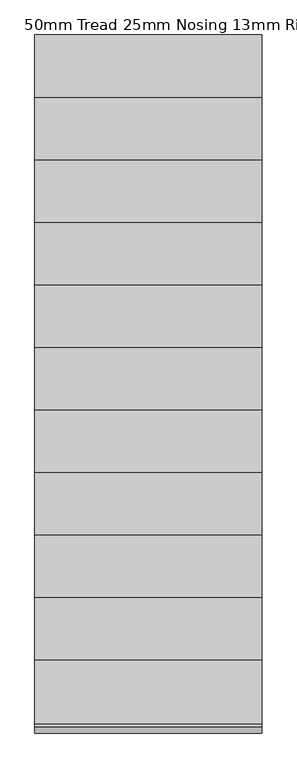
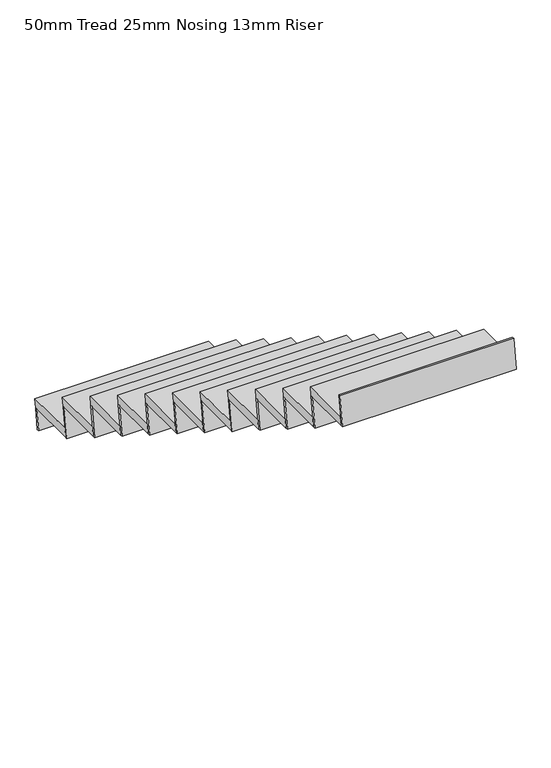
"""IFC4 building model written with IfcOpenShell, lengths in millimetres: stair flight geometry, 50mm Tread 25mm Nosing 13mm Riser."""

from ifc_helpers import new_model, si_unit, frame, origin, place, context, project, spatial, polyline, outline, extrude, source, transform, mapped, element, save


def stair_flight_50mm_tread_25mm_nosing_13mm_riser_4d1d0ec9(model_context):
    return source(origin(), model_context, "Body", "SweptSolid", [
        extrude(outline(polyline([(58.5943271, 173.9130435), (358.5943271, 173.9130435), (351.4068271, 123.9130435), (51.4068271, 123.9130435), (58.5943271, 173.9130435)])), frame((-1692.5284847, 0.0, 0.0), z_axis=(1.0, 0.0, 0.0), x_axis=(0.0, 1.0, 0.0)), (0.0, 0.0, 1.0), 1000.0257812),
        extrude(outline(polyline([(351.4068271, 123.9130435), (333.5943271, 0.0), (320.9658371, 0.0), (338.7783371, 123.9130435), (351.4068271, 123.9130435)])), frame((-1692.5284847, 0.0, 0.0), z_axis=(1.0, 0.0, 0.0), x_axis=(0.0, 1.0, 0.0)), (0.0, 0.0, 1.0), 1000.0257812),
        extrude(outline(polyline([(76.4068271, 297.826087), (51.4068271, 123.9130435), (38.7783371, 123.9130435), (63.7783371, 297.826087), (76.4068271, 297.826087)])), frame((-1692.5284847, 0.0, 0.0), z_axis=(1.0, 0.0, 0.0), x_axis=(0.0, 1.0, 0.0)), (0.0, 0.0, 1.0), 1000.0257813),
        extrude(outline(polyline([(-216.4056729, 347.826087), (83.5943271, 347.826087), (76.4068271, 297.826087), (-223.5931729, 297.826087), (-216.4056729, 347.826087)])), frame((-1692.5284847, 0.0, 0.0), z_axis=(1.0, 0.0, 0.0), x_axis=(0.0, 1.0, 0.0)), (0.0, 0.0, 1.0), 1000.0257812),
        extrude(outline(polyline([(-198.5931729, 471.7391304), (-223.5931729, 297.826087), (-236.2216629, 297.826087), (-211.2216629, 471.7391304), (-198.5931729, 471.7391304)])), frame((-1692.5284847, 0.0, 0.0), z_axis=(1.0, 0.0, 0.0), x_axis=(0.0, 1.0, 0.0)), (0.0, 0.0, 1.0), 1000.0257813),
        extrude(outline(polyline([(-491.4056729, 521.7391304), (-191.4056729, 521.7391304), (-198.5931729, 471.7391304), (-498.5931729, 471.7391304), (-491.4056729, 521.7391304)])), frame((-1692.5284847, 0.0, 0.0), z_axis=(1.0, 0.0, 0.0), x_axis=(0.0, 1.0, 0.0)), (0.0, 0.0, 1.0), 1000.0257813),
        extrude(outline(polyline([(-473.5931729, 645.6521739), (-498.5931729, 471.7391304), (-511.2216629, 471.7391304), (-486.2216629, 645.6521739), (-473.5931729, 645.6521739)])), frame((-1692.5284847, 0.0, 0.0), z_axis=(1.0, 0.0, 0.0), x_axis=(0.0, 1.0, 0.0)), (0.0, 0.0, 1.0), 1000.0257813),
        extrude(outline(polyline([(-766.4056729, 695.6521739), (-466.4056729, 695.6521739), (-473.5931729, 645.6521739), (-773.5931729, 645.6521739), (-766.4056729, 695.6521739)])), frame((-1692.5284847, 0.0, 0.0), z_axis=(1.0, 0.0, 0.0), x_axis=(0.0, 1.0, 0.0)), (0.0, 0.0, 1.0), 1000.0257813),
        extrude(outline(polyline([(-748.5931729, 819.5652174), (-773.5931729, 645.6521739), (-786.2216629, 645.6521739), (-761.2216629, 819.5652174), (-748.5931729, 819.5652174)])), frame((-1692.5284847, 0.0, 0.0), z_axis=(1.0, 0.0, 0.0), x_axis=(0.0, 1.0, 0.0)), (0.0, 0.0, 1.0), 1000.0257813),
        extrude(outline(polyline([(-1041.4056729, 869.5652174), (-741.4056729, 869.5652174), (-748.5931729, 819.5652174), (-1048.5931729, 819.5652174), (-1041.4056729, 869.5652174)])), frame((-1692.5284847, 0.0, 0.0), z_axis=(1.0, 0.0, 0.0), x_axis=(0.0, 1.0, 0.0)), (0.0, 0.0, 1.0), 1000.0257813),
        extrude(outline(polyline([(-1023.5931729, 993.4782609), (-1048.5931729, 819.5652174), (-1061.2216629, 819.5652174), (-1036.2216629, 993.4782609), (-1023.5931729, 993.4782609)])), frame((-1692.5284847, 0.0, 0.0), z_axis=(1.0, 0.0, 0.0), x_axis=(0.0, 1.0, 0.0)), (0.0, 0.0, 1.0), 1000.0257813),
        extrude(outline(polyline([(-1316.4056729, 1043.4782609), (-1016.4056729, 1043.4782609), (-1023.5931729, 993.4782609), (-1323.5931729, 993.4782609), (-1316.4056729, 1043.4782609)])), frame((-1692.5284847, 0.0, 0.0), z_axis=(1.0, 0.0, 0.0), x_axis=(0.0, 1.0, 0.0)), (0.0, 0.0, 1.0), 1000.0257813),
        extrude(outline(polyline([(-1298.5931729, 1167.3913043), (-1323.5931729, 993.4782609), (-1336.2216629, 993.4782609), (-1311.2216629, 1167.3913043), (-1298.5931729, 1167.3913043)])), frame((-1692.5284847, 0.0, 0.0), z_axis=(1.0, 0.0, 0.0), x_axis=(0.0, 1.0, 0.0)), (0.0, 0.0, 1.0), 1000.0257813),
        extrude(outline(polyline([(-1591.4056729, 1217.3913043), (-1291.4056729, 1217.3913043), (-1298.5931729, 1167.3913043), (-1598.5931729, 1167.3913043), (-1591.4056729, 1217.3913043)])), frame((-1692.5284847, 0.0, 0.0), z_axis=(1.0, 0.0, 0.0), x_axis=(0.0, 1.0, 0.0)), (0.0, 0.0, 1.0), 1000.0257813),
        extrude(outline(polyline([(-1573.5931729, 1341.3043478), (-1598.5931729, 1167.3913043), (-1611.2216629, 1167.3913043), (-1586.2216629, 1341.3043478), (-1573.5931729, 1341.3043478)])), frame((-1692.5284847, 0.0, 0.0), z_axis=(1.0, 0.0, 0.0), x_axis=(0.0, 1.0, 0.0)), (0.0, 0.0, 1.0), 1000.0257813),
        extrude(outline(polyline([(-1866.4056729, 1391.3043478), (-1566.4056729, 1391.3043478), (-1573.5931729, 1341.3043478), (-1873.5931729, 1341.3043478), (-1866.4056729, 1391.3043478)])), frame((-1692.5284847, 0.0, 0.0), z_axis=(1.0, 0.0, 0.0), x_axis=(0.0, 1.0, 0.0)), (0.0, 0.0, 1.0), 1000.0257813),
        extrude(outline(polyline([(-1848.5931729, 1515.2173913), (-1873.5931729, 1341.3043478), (-1886.2216629, 1341.3043478), (-1861.2216629, 1515.2173913), (-1848.5931729, 1515.2173913)])), frame((-1692.5284847, 0.0, 0.0), z_axis=(1.0, 0.0, 0.0), x_axis=(0.0, 1.0, 0.0)), (0.0, 0.0, 1.0), 1000.0257813),
        extrude(outline(polyline([(-2141.4056729, 1565.2173913), (-1841.4056729, 1565.2173913), (-1848.5931729, 1515.2173913), (-2148.5931729, 1515.2173913), (-2141.4056729, 1565.2173913)])), frame((-1692.5284847, 0.0, 0.0), z_axis=(1.0, 0.0, 0.0), x_axis=(0.0, 1.0, 0.0)), (0.0, 0.0, 1.0), 1000.0257813),
        extrude(outline(polyline([(-2123.5931729, 1689.1304348), (-2148.5931729, 1515.2173913), (-2161.2216629, 1515.2173913), (-2136.2216629, 1689.1304348), (-2123.5931729, 1689.1304348)])), frame((-1692.5284847, 0.0, 0.0), z_axis=(1.0, 0.0, 0.0), x_axis=(0.0, 1.0, 0.0)), (0.0, 0.0, 1.0), 1000.0257813),
        extrude(outline(polyline([(-2416.4056729, 1739.1304348), (-2116.4056729, 1739.1304348), (-2123.5931729, 1689.1304348), (-2423.5931729, 1689.1304348), (-2416.4056729, 1739.1304348)])), frame((-1692.5284847, 0.0, 0.0), z_axis=(1.0, 0.0, 0.0), x_axis=(0.0, 1.0, 0.0)), (0.0, 0.0, 1.0), 1000.0257813),
        extrude(outline(polyline([(-2398.5931729, 1863.0434783), (-2423.5931729, 1689.1304348), (-2436.2216629, 1689.1304348), (-2411.2216629, 1863.0434783), (-2398.5931729, 1863.0434783)])), frame((-1692.5284847, 0.0, 0.0), z_axis=(1.0, 0.0, 0.0), x_axis=(0.0, 1.0, 0.0)), (0.0, 0.0, 1.0), 1000.0257813),
        extrude(outline(polyline([(-2673.5931729, 2036.9565217), (-2698.5931729, 1863.0434783), (-2711.2216629, 1863.0434783), (-2686.2216629, 2036.9565217), (-2673.5931729, 2036.9565217)])), frame((-1692.5284847, 0.0, 0.0), z_axis=(1.0, 0.0, 0.0), x_axis=(0.0, 1.0, 0.0)), (0.0, 0.0, 1.0), 1000.0257812),
        extrude(outline(polyline([(-2691.4056729, 1913.0434783), (-2391.4056729, 1913.0434783), (-2398.5931729, 1863.0434783), (-2698.5931729, 1863.0434783), (-2691.4056729, 1913.0434783)])), frame((-1692.5284847, 0.0, 0.0), z_axis=(1.0, 0.0, 0.0), x_axis=(0.0, 1.0, 0.0)), (0.0, 0.0, 1.0), 1000.0257813),
    ])


if __name__ == "__main__":
    model = new_model("IFC4")
    model_context = context("Model", 3, world=origin())
    ifc_project = project(units=[si_unit("LENGTHUNIT", "METRE", prefix="MILLI")], contexts=[model_context])
    site = spatial("IfcSite", under=ifc_project)
    building = spatial("IfcBuilding", under=site)
    placement = place(None, origin())
    stair_flight_50mm_tread_25mm_nosing_13mm_riser_shape = stair_flight_50mm_tread_25mm_nosing_13mm_riser_4d1d0ec9(model_context)
    element("IfcStairFlight", 1, ObjectType="50mm Tread 25mm Nosing 13mm Riser", at=placement, inside=building, context=model_context, shape_type="MappedRepresentation", body=[
        mapped(stair_flight_50mm_tread_25mm_nosing_13mm_riser_shape, transform((0.0, 0.0, 0.0), x_axis=(1.0, 0.0, 0.0), y_axis=(0.0, 1.0, 0.0), z_axis=(0.0, 0.0, 1.0))),
    ])
    save(model, "model.ifc")
